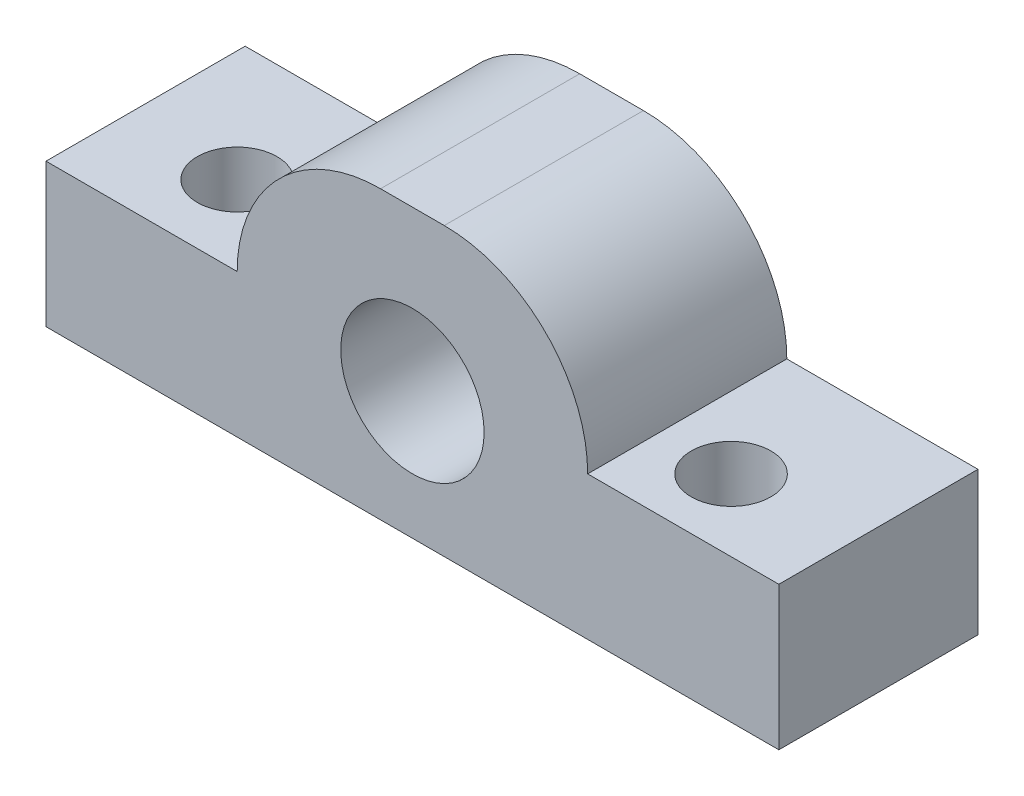
from build123d import *

# Parameters (mm, degrees)
PILLOW_BLOCK_PROFILE_R  = 9
PILLOW_BLOCK_BODY_DEPTH = 12.5
MOUNTING_HOLES_2X_10_D  = 10


with BuildPart() as part:
    # Pillow Block Profile → Pillow Block Body (new, symmetric)
    with BuildSketch(Plane.XY):
        with BuildLine():
            Line((46, 0), (-46, 0))
            Line((-46, 0), (-46, 18))
            Line((-46, 18), (-22, 18))
            ThreePointArc((-22, 18), (-16.727922061, 30.727922061), (-4, 36))
            Line((-4, 36), (4, 36))
            ThreePointArc((4, 36), (16.727922061, 30.727922061), (22, 18))
            Line((22, 18), (46, 18))
            Line((46, 18), (46, 0))
        make_face()
        with Locations((0, 16)):
            Circle(PILLOW_BLOCK_PROFILE_R, mode=Mode.SUBTRACT)
    extrude(amount=PILLOW_BLOCK_BODY_DEPTH, both=True)

    # Mounting Holes 2xØ10 (through all)
    with Locations(Plane(origin=(-32, 18, 2.5), x_dir=(1, 0, 0), z_dir=(0, 1, 0))):
        with Locations((0, 0), (63, -1)):
            Hole(MOUNTING_HOLES_2X_10_D / 2)


solid = part.part
